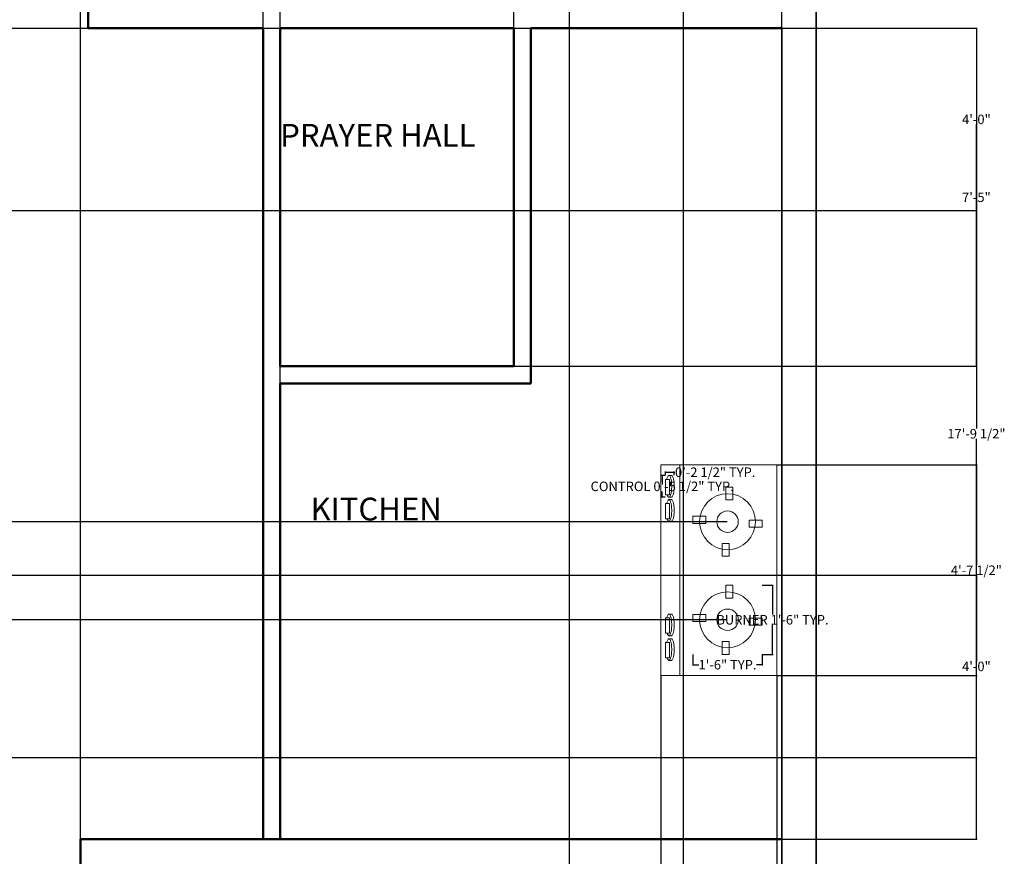
# Model space of a CAD drawing. Units: inches. Extents: x 594 to 1173, y 353 to 1285.
# Tile 5 of 6: x 914 to 1173, y 844 to 1065. Entities that reach past the tile are written whole.
import ezdxf

# ---------------------------------------------------------------- set-up
doc = ezdxf.new("R2010")
doc.units = ezdxf.units.IN
doc.header["$MEASUREMENT"] = 0
for name, color, linetype, lineweight in [('A-ANNO-DIMS', 2, 'Continuous', 18), ('A-AREA-IDEN', 7, 'Continuous', 25), ('A-EQPM', 8, 'Continuous', 18), ('A-WALL', 7, 'Continuous', 50), ('C-PROP', 7, 'Continuous', 35)]:
    doc.layers.add(name, color=color, linetype=linetype, lineweight=lineweight)
doc.styles.get("Standard").update_dxf_attribs({"font": 'arial.ttf'})
doc.dimstyles.get("Standard").update_dxf_attribs({"dimtxt": 2.5, "dimasz": 0.18, "dimexe": 0.18, "dimexo": 0.0625, "dimgap": 0.09, "dimtad": 0, "dimtih": 1, "dimtoh": 1, "dimzin": 0, "dimdsep": 46, "dimlunit": 3, "dimtxsty": 'Standard', "dimcen": 0.09, "dimadec": 0, "dimazin": 0, "dimtfac": 1, "dimtofl": 0, "dimtmove": 0, "dimatfit": 3, "dimfxl": 1, "dimtolj": 1, "dimtzin": 0, "dimarcsym": 0})

# ---------------------------------------------------------------- blocks, each defined once
blk = doc.blocks.new('COOKTOP-BURNER')
for p, q in [((-0.44, 9.1), (-0.44, 5.73)), ((1.43, 9.1), (-0.44, 9.1)), ((1.43, 5.73), (1.43, 9.1)), ((-0.44, 5.73), (1.43, 5.73)), ((-5.73, 1.43), (-9.1, 1.43)), ((-9.1, 1.43), (-9.1, -0.44)), ((-5.73, -0.44), (-5.73, 1.43)), ((5.73, 0.44), (5.73, -1.43)), ((9.1, 0.44), (5.73, 0.44)), ((9.1, -1.43), (9.1, 0.44)), ((-9.1, -0.44), (-5.73, -0.44)), ((5.73, -1.43), (9.1, -1.43)), ((-1.43, -5.73), (-1.43, -9.1)), ((0.44, -5.73), (-1.43, -5.73)), ((0.44, -9.1), (0.44, -5.73)), ((-1.43, -9.1), (0.44, -9.1))]:
    blk.add_line(p, q)
for radius in [7.35, 2.82]:
    blk.add_circle((0, 0), radius)
blk = doc.blocks.new('COOKTOP-CONTROL-KNOB')
for p, q in [((1.55, 5.72), (0.9, 5.72)), ((0, 0.65), (0, 4.69)), ((0, 4.69), (1.04, 4.69)), ((1.04, 4.69), (1.04, 0.65)), ((1.04, 0.65), (0, 0.65)), ((1.63, 0), (0.9, 0.01))]:
    blk.add_line(p, q)
for centre, radius, start, end in [((2.87, 4.24), 2.58, 148.0894, 165.5369), ((0.9, 5.47), 0.251, 90, 148.0894), ((0.9, 5.47), 0.251, 31.9106, 90), ((-1.08, 4.24), 2.58, 14.4631, 31.9106), ((1.55, 5.47), 0.251, 31.9106, 90), ((-0.42, 4.24), 2.58, 14.4631, 31.9106), ((6.08, 3.42), 5.89, 165.5369, 167.5389), ((-4.28, 3.42), 5.89, 6.0983, 14.4631), ((-9.43, 2.87), 11.07, 0, 6.0983), ((-9.43, 2.87), 11.07, 353.9017, 0), ((-3.62, 3.42), 5.89, 6.0983, 14.4631), ((-8.78, 2.87), 11.07, 0, 6.0983), ((-8.78, 2.87), 11.07, 353.9017, 0), ((2.87, 1.49), 2.58, 198.9155, 211.9106), ((0.9, 0.26), 0.251, 211.9106, 270), ((0.9, 0.26), 0.251, 270, 328.0894), ((-1.08, 1.49), 2.58, 328.0894, 345.5369), ((-4.28, 2.31), 5.89, 345.5369, 353.9017), ((1.55, 0.26), 0.251, 252.0546, 270), ((1.55, 0.26), 0.251, 270, 328.0894), ((-0.42, 1.49), 2.58, 328.0894, 345.5369), ((-3.62, 2.31), 5.89, 345.5369, 353.9017)]:
    blk.add_arc(centre, radius, start, end)
blk = doc.blocks.new('*D34')
at = {"layer": 'A-ANNO-DIMS', "color": 0, "lineweight": -2, "transparency": 16777216}
for p, q in [((1109.21, 915.65), (1112.06, 915.65)), ((1111.88, 915.47), (1111.88, 907.92)), ((1111.88, 897.63), (1111.88, 905.19)), ((1109.21, 897.45), (1112.06, 897.45))]:
    blk.add_line(p, q, dxfattribs=at)
at = {"layer": 'A-ANNO-DIMS', "color": 0, "transparency": 16777216}
for points in [[(1111.85, 915.47), (1111.91, 915.47), (1111.88, 915.65)], [(1111.85, 897.63), (1111.91, 897.63), (1111.88, 897.45)]]:
    blk.add_solid(points, dxfattribs=at)
at = {"layer": 'Defpoints', "color": 0, "transparency": 16777216}
for p in [(1109.15, 915.65), (1111.88, 915.65), (1109.15, 897.45)]:
    blk.add_point(p, dxfattribs=at)
at = {"layer": 'A-ANNO-DIMS', "color": 0, "transparency": 16777216, "insert": (1111.88, 906.55), "char_height": 2.5, "attachment_point": 5}
blk.add_mtext('\\A1;BURNER 1\'-6" TYP.', dxfattribs=at)
blk = doc.blocks.new('*D35')
at = {"layer": 'A-ANNO-DIMS', "color": 0, "lineweight": -2, "transparency": 16777216}
for p, q in [((1090.95, 897.39), (1090.95, 894.54)), ((1109.15, 897.39), (1109.15, 894.54)), ((1091.13, 894.72), (1092.46, 894.72)), ((1108.97, 894.72), (1107.64, 894.72))]:
    blk.add_line(p, q, dxfattribs=at)
at = {"layer": 'A-ANNO-DIMS', "color": 0, "transparency": 16777216}
for points in [[(1091.13, 894.75), (1091.13, 894.69), (1090.95, 894.72)], [(1108.97, 894.75), (1108.97, 894.69), (1109.15, 894.72)]]:
    blk.add_solid(points, dxfattribs=at)
at = {"layer": 'Defpoints', "color": 0, "transparency": 16777216}
for p in [(1090.95, 897.45), (1109.15, 897.45), (1109.15, 894.72)]:
    blk.add_point(p, dxfattribs=at)
at = {"layer": 'A-ANNO-DIMS', "color": 0, "transparency": 16777216, "insert": (1100.05, 894.72), "char_height": 2.5, "attachment_point": 5}
blk.add_mtext('\\A1;1\'-6" TYP.', dxfattribs=at)
blk = doc.blocks.new('*D36')
at = {"layer": 'A-ANNO-DIMS', "color": 0, "lineweight": -2, "transparency": 16777216}
for p, q in [((1083.66, 944.54), (1082.68, 944.54)), ((1082.86, 944.36), (1082.86, 943.07)), ((1083.66, 938.82), (1082.68, 938.82)), ((1082.86, 939), (1082.86, 940.3))]:
    blk.add_line(p, q, dxfattribs=at)
at = {"layer": 'A-ANNO-DIMS', "color": 0, "transparency": 16777216}
for points in [[(1082.83, 944.36), (1082.89, 944.36), (1082.86, 944.54)], [(1082.83, 939), (1082.89, 939), (1082.86, 938.82)]]:
    blk.add_solid(points, dxfattribs=at)
at = {"layer": 'Defpoints', "color": 0, "transparency": 16777216}
for p in [(1082.86, 944.54), (1083.72, 944.54), (1083.72, 938.82)]:
    blk.add_point(p, dxfattribs=at)
at = {"layer": 'A-ANNO-DIMS', "color": 0, "transparency": 16777216, "insert": (1082.86, 941.68), "char_height": 2.5, "attachment_point": 5}
blk.add_mtext('\\A1;CONTROL 0\'-5 1/2" TYP.', dxfattribs=at)
blk = doc.blocks.new('*D37')
at = {"layer": 'A-ANNO-DIMS', "color": 0, "lineweight": -2, "transparency": 16777216}
for p, q in [((1083.72, 944.61), (1083.72, 945.58)), ((1083.9, 945.4), (1085.83, 945.4)), ((1086.01, 944.61), (1086.01, 945.58)), ((1086.01, 945.4), (1086.19, 945.4))]:
    blk.add_line(p, q, dxfattribs=at)
at = {"layer": 'A-ANNO-DIMS', "color": 0, "transparency": 16777216}
for points in [[(1083.9, 945.43), (1083.9, 945.37), (1083.72, 945.4)], [(1085.83, 945.43), (1085.83, 945.37), (1086.01, 945.4)]]:
    blk.add_solid(points, dxfattribs=at)
at = {"layer": 'Defpoints', "color": 0, "transparency": 16777216}
for p in [(1083.72, 944.54), (1086.01, 945.4), (1086.01, 944.54)]:
    blk.add_point(p, dxfattribs=at)
at = {"layer": 'A-ANNO-DIMS', "color": 0, "transparency": 16777216, "insert": (1096.81, 945.4), "char_height": 2.5, "attachment_point": 5}
blk.add_mtext('\\A1;0\'-2 1/2" TYP.', dxfattribs=at)
blk = doc.blocks.new('*D52')
at = {"layer": 'A-ANNO-DIMS', "color": 0, "lineweight": -2, "transparency": 16777216}
for p, q in [((982.34, 968.85), (982.34, 1281.16)), ((982.52, 1280.98), (1044.07, 1280.98)), ((1114.16, 1280.98), (1052.6, 1280.98)), ((1114.34, 848.85), (1114.34, 1281.16))]:
    blk.add_line(p, q, dxfattribs=at)
at = {"layer": 'A-ANNO-DIMS', "color": 0, "transparency": 16777216}
for points in [[(982.52, 1281.01), (982.52, 1280.95), (982.34, 1280.98)], [(1114.16, 1281.01), (1114.16, 1280.95), (1114.34, 1280.98)]]:
    blk.add_solid(points, dxfattribs=at)
at = {"layer": 'Defpoints', "color": 0, "transparency": 16777216}
for p in [(1114.34, 1280.98), (982.34, 968.78), (1114.34, 848.78)]:
    blk.add_point(p, dxfattribs=at)
at = {"layer": 'A-ANNO-DIMS', "color": 0, "transparency": 16777216, "insert": (1048.34, 1280.98), "char_height": 2.5, "attachment_point": 5}
blk.add_mtext('\\A1;11\'-0"', dxfattribs=at)
blk = doc.blocks.new('*D53')
at = {"layer": 'A-ANNO-DIMS', "color": 0, "lineweight": -2, "transparency": 16777216}
for p, q in [((1114.4, 1062.28), (1165.72, 1062.28)), ((1165.54, 1062.1), (1165.54, 956.92)), ((1165.54, 848.96), (1165.54, 954.15)), ((1114.4, 848.78), (1165.72, 848.78))]:
    blk.add_line(p, q, dxfattribs=at)
at = {"layer": 'A-ANNO-DIMS', "color": 0, "transparency": 16777216}
for points in [[(1165.51, 1062.1), (1165.57, 1062.1), (1165.54, 1062.28)], [(1165.51, 848.96), (1165.57, 848.96), (1165.54, 848.78)]]:
    blk.add_solid(points, dxfattribs=at)
at = {"layer": 'Defpoints', "color": 0, "transparency": 16777216}
for p in [(1114.34, 1062.28), (1165.54, 1062.28), (1114.34, 848.78)]:
    blk.add_point(p, dxfattribs=at)
at = {"layer": 'A-ANNO-DIMS', "color": 0, "transparency": 16777216, "insert": (1165.54, 955.53), "char_height": 2.5, "attachment_point": 5}
blk.add_mtext('\\A1;17\'-9 1/2"', dxfattribs=at)
blk = doc.blocks.new('*D54')
at = {"layer": 'A-ANNO-DIMS', "color": 0, "lineweight": -2, "transparency": 16777216}
for p, q in [((982.34, 1062.35), (982.34, 1281.16)), ((982.52, 1280.98), (1006.76, 1280.98)), ((1043.66, 1280.98), (1019.41, 1280.98)), ((1043.84, 1062.35), (1043.84, 1281.16))]:
    blk.add_line(p, q, dxfattribs=at)
at = {"layer": 'A-ANNO-DIMS', "color": 0, "transparency": 16777216}
for points in [[(982.52, 1281.01), (982.52, 1280.95), (982.34, 1280.98)], [(1043.66, 1281.01), (1043.66, 1280.95), (1043.84, 1280.98)]]:
    blk.add_solid(points, dxfattribs=at)
at = {"layer": 'Defpoints', "color": 0, "transparency": 16777216}
for p in [(1043.84, 1280.98), (982.34, 1062.28), (1043.84, 1062.28)]:
    blk.add_point(p, dxfattribs=at)
at = {"layer": 'A-ANNO-DIMS', "color": 0, "transparency": 16777216, "insert": (1013.09, 1280.98), "char_height": 2.5, "attachment_point": 5}
blk.add_mtext('\\A1;5\'-1 1/2"', dxfattribs=at)
blk = doc.blocks.new('*D55')
at = {"layer": 'A-ANNO-DIMS', "color": 0, "lineweight": -2, "transparency": 16777216}
for p, q in [((1043.9, 1062.28), (1165.72, 1062.28)), ((1165.54, 1062.1), (1165.54, 1019.14)), ((1165.54, 973.46), (1165.54, 1016.42)), ((1043.9, 973.28), (1165.72, 973.28))]:
    blk.add_line(p, q, dxfattribs=at)
at = {"layer": 'A-ANNO-DIMS', "color": 0, "transparency": 16777216}
for points in [[(1165.51, 1062.1), (1165.57, 1062.1), (1165.54, 1062.28)], [(1165.51, 973.46), (1165.57, 973.46), (1165.54, 973.28)]]:
    blk.add_solid(points, dxfattribs=at)
at = {"layer": 'Defpoints', "color": 0, "transparency": 16777216}
for p in [(1043.84, 1062.28), (1165.54, 1062.28), (1043.84, 973.28)]:
    blk.add_point(p, dxfattribs=at)
at = {"layer": 'A-ANNO-DIMS', "color": 0, "transparency": 16777216, "insert": (1165.54, 1017.78), "char_height": 2.5, "attachment_point": 5}
blk.add_mtext('\\A1;7\'-5"', dxfattribs=at)
blk = doc.blocks.new('*D58')
at = {"layer": 'A-ANNO-DIMS', "color": 0, "lineweight": -2, "transparency": 16777216}
for p, q in [((829.34, 647.85), (829.34, 1281.16)), ((829.52, 1280.98), (873.26, 1280.98)), ((929.66, 1280.98), (885.91, 1280.98)), ((929.84, 647.85), (929.84, 1281.16))]:
    blk.add_line(p, q, dxfattribs=at)
at = {"layer": 'A-ANNO-DIMS', "color": 0, "transparency": 16777216}
for points in [[(829.52, 1281.01), (829.52, 1280.95), (829.34, 1280.98)], [(929.66, 1281.01), (929.66, 1280.95), (929.84, 1280.98)]]:
    blk.add_solid(points, dxfattribs=at)
at = {"layer": 'Defpoints', "color": 0, "transparency": 16777216}
for p in [(929.84, 1280.98), (829.34, 647.78), (929.84, 647.78)]:
    blk.add_point(p, dxfattribs=at)
at = {"layer": 'A-ANNO-DIMS', "color": 0, "transparency": 16777216, "insert": (879.59, 1280.98), "char_height": 2.5, "attachment_point": 5}
blk.add_mtext('\\A1;8\'-4 1/2"', dxfattribs=at)
blk = doc.blocks.new('*D61')
at = {"layer": 'A-ANNO-DIMS', "color": 0, "lineweight": -2, "transparency": 16777216}
for p, q in [((728.84, 1062.35), (728.84, 1281.16)), ((729.02, 1280.98), (848.93, 1280.98)), ((977.66, 1280.98), (857.74, 1280.98)), ((977.84, 1062.35), (977.84, 1281.16))]:
    blk.add_line(p, q, dxfattribs=at)
at = {"layer": 'A-ANNO-DIMS', "color": 0, "transparency": 16777216}
for points in [[(729.02, 1281.01), (729.02, 1280.95), (728.84, 1280.98)], [(977.66, 1281.01), (977.66, 1280.95), (977.84, 1280.98)]]:
    blk.add_solid(points, dxfattribs=at)
at = {"layer": 'Defpoints', "color": 0, "transparency": 16777216}
for p in [(977.84, 1280.98), (728.84, 1062.28), (977.84, 1062.28)]:
    blk.add_point(p, dxfattribs=at)
at = {"layer": 'A-ANNO-DIMS', "color": 0, "transparency": 16777216, "insert": (853.34, 1280.98), "char_height": 2.5, "attachment_point": 5}
blk.add_mtext('\\A1;20\'-9"', dxfattribs=at)
blk = doc.blocks.new('*D62')
at = {"layer": 'A-ANNO-DIMS', "color": 0, "lineweight": -2, "transparency": 16777216}
for p, q in [((1082.5, 891.79), (1082.5, 356.4)), ((1113.01, 891.79), (1113.01, 356.4)), ((1082.68, 356.58), (1091.41, 356.58)), ((1112.83, 356.58), (1104.1, 356.58))]:
    blk.add_line(p, q, dxfattribs=at)
at = {"layer": 'A-ANNO-DIMS', "color": 0, "transparency": 16777216}
for points in [[(1082.68, 356.61), (1082.68, 356.55), (1082.5, 356.58)], [(1112.83, 356.61), (1112.83, 356.55), (1113.01, 356.58)]]:
    blk.add_solid(points, dxfattribs=at)
at = {"layer": 'Defpoints', "color": 0, "transparency": 16777216}
for p in [(1082.5, 891.85), (1113.01, 891.85), (1113.01, 356.58)]:
    blk.add_point(p, dxfattribs=at)
at = {"layer": 'A-ANNO-DIMS', "color": 0, "transparency": 16777216, "insert": (1097.75, 356.58), "char_height": 2.5, "attachment_point": 5}
blk.add_mtext('\\A1;2\'-6 1/2"', dxfattribs=at)
blk = doc.blocks.new('*D63')
at = {"layer": 'A-ANNO-DIMS', "color": 0, "lineweight": -2, "transparency": 16777216}
for p, q in [((1113.07, 947.33), (1165.72, 947.33)), ((1165.54, 947.15), (1165.54, 920.97)), ((1165.54, 892.03), (1165.54, 918.21)), ((1113.07, 891.85), (1165.72, 891.85))]:
    blk.add_line(p, q, dxfattribs=at)
at = {"layer": 'A-ANNO-DIMS', "color": 0, "transparency": 16777216}
for points in [[(1165.51, 947.15), (1165.57, 947.15), (1165.54, 947.33)], [(1165.51, 892.03), (1165.57, 892.03), (1165.54, 891.85)]]:
    blk.add_solid(points, dxfattribs=at)
at = {"layer": 'Defpoints', "color": 0, "transparency": 16777216}
for p in [(1113.01, 947.33), (1165.54, 947.33), (1113.01, 891.85)]:
    blk.add_point(p, dxfattribs=at)
at = {"layer": 'A-ANNO-DIMS', "color": 0, "transparency": 16777216, "insert": (1165.54, 919.59), "char_height": 2.5, "attachment_point": 5}
blk.add_mtext('\\A1;4\'-7 1/2"', dxfattribs=at)
blk = doc.blocks.new('*D67')
at = {"layer": 'A-ANNO-DIMS', "color": 0, "lineweight": -2, "transparency": 16777216}
for p, q in [((1058.34, 1093.22), (1058.34, 356.4)), ((1088.34, 1093.22), (1088.34, 356.4)), ((1058.52, 356.58), (1069.9, 356.58)), ((1088.16, 356.58), (1076.77, 356.58))]:
    blk.add_line(p, q, dxfattribs=at)
at = {"layer": 'A-ANNO-DIMS', "color": 0, "transparency": 16777216}
for points in [[(1058.52, 356.61), (1058.52, 356.55), (1058.34, 356.58)], [(1088.16, 356.61), (1088.16, 356.55), (1088.34, 356.58)]]:
    blk.add_solid(points, dxfattribs=at)
at = {"layer": 'Defpoints', "color": 0, "transparency": 16777216}
for p in [(1058.34, 1093.28), (1088.34, 1093.28), (1058.34, 356.58)]:
    blk.add_point(p, dxfattribs=at)
at = {"layer": 'A-ANNO-DIMS', "color": 0, "transparency": 16777216, "insert": (1073.34, 356.58), "char_height": 2.5, "attachment_point": 5}
blk.add_mtext('\\A1;2\'-6"', dxfattribs=at)
blk = doc.blocks.new('*D71')
at = {"layer": 'A-ANNO-DIMS', "color": 0, "lineweight": -2, "transparency": 16777216}
for p, q in [((812.9, 918.28), (1165.72, 918.28)), ((1165.54, 918.1), (1165.54, 895.65)), ((1165.54, 870.46), (1165.54, 892.92)), ((812.9, 870.28), (1165.72, 870.28))]:
    blk.add_line(p, q, dxfattribs=at)
at = {"layer": 'A-ANNO-DIMS', "color": 0, "transparency": 16777216}
for points in [[(1165.51, 918.1), (1165.57, 918.1), (1165.54, 918.28)], [(1165.51, 870.46), (1165.57, 870.46), (1165.54, 870.28)]]:
    blk.add_solid(points, dxfattribs=at)
at = {"layer": 'Defpoints', "color": 0, "transparency": 16777216}
for p in [(812.84, 918.28), (1165.54, 918.28), (812.84, 870.28)]:
    blk.add_point(p, dxfattribs=at)
at = {"layer": 'A-ANNO-DIMS', "color": 0, "transparency": 16777216, "insert": (1165.54, 894.28), "char_height": 2.5, "attachment_point": 5}
blk.add_mtext('\\A1;4\'-0"', dxfattribs=at)
blk = doc.blocks.new('*D74')
at = {"layer": 'A-ANNO-DIMS', "color": 0, "lineweight": -2, "transparency": 16777216}
for p, q in [((812.9, 1062.28), (1165.72, 1062.28)), ((1165.54, 1062.1), (1165.54, 1039.65)), ((1165.54, 1014.46), (1165.54, 1036.92)), ((812.9, 1014.28), (1165.72, 1014.28))]:
    blk.add_line(p, q, dxfattribs=at)
at = {"layer": 'A-ANNO-DIMS', "color": 0, "transparency": 16777216}
for points in [[(1165.51, 1062.1), (1165.57, 1062.1), (1165.54, 1062.28)], [(1165.51, 1014.46), (1165.57, 1014.46), (1165.54, 1014.28)]]:
    blk.add_solid(points, dxfattribs=at)
at = {"layer": 'Defpoints', "color": 0, "transparency": 16777216}
for p in [(812.84, 1062.28), (1165.54, 1062.28), (812.84, 1014.28)]:
    blk.add_point(p, dxfattribs=at)
at = {"layer": 'A-ANNO-DIMS', "color": 0, "transparency": 16777216, "insert": (1165.54, 1038.28), "char_height": 2.5, "attachment_point": 5}
blk.add_mtext('\\A1;4\'-0"', dxfattribs=at)
blk = doc.blocks.new('*D79')
at = {"layer": 'A-ANNO-DIMS', "color": 0, "lineweight": -2, "transparency": 16777216}
for p, q in [((1099.99, 932.38), (600.96, 932.38)), ((601.14, 932.2), (601.14, 920.81)), ((601.14, 906.73), (601.14, 918.12)), ((1099.99, 906.55), (600.96, 906.55))]:
    blk.add_line(p, q, dxfattribs=at)
at = {"layer": 'A-ANNO-DIMS', "color": 0, "transparency": 16777216}
for points in [[(601.11, 932.2), (601.17, 932.2), (601.14, 932.38)], [(601.11, 906.73), (601.17, 906.73), (601.14, 906.55)]]:
    blk.add_solid(points, dxfattribs=at)
at = {"layer": 'Defpoints', "color": 0, "transparency": 16777216}
for p in [(601.14, 932.38), (1100.05, 932.38), (1100.05, 906.55)]:
    blk.add_point(p, dxfattribs=at)
at = {"layer": 'A-ANNO-DIMS', "color": 0, "transparency": 16777216, "insert": (601.14, 919.47), "char_height": 2.5, "attachment_point": 5}
blk.add_mtext('\\A1;2\'-2"', dxfattribs=at)

msp = doc.modelspace()

# ---------------------------------------------------------------- linework, layer by layer
at = {"layer": 'A-EQPM'}
for p, q in [((1082.501, 947.329), (1113.008, 947.329)), ((1082.501, 891.849), (1082.501, 947.329)), ((1087.463, 891.849), (1087.463, 947.329)), ((1113.008, 947.329), (1113.008, 891.849)), ((1113.008, 891.849), (1082.501, 891.849))]:
    msp.add_line(p, q, dxfattribs=at)
at = {"layer": 'A-WALL'}
for p, q in [((931.837, 1062.283), (931.837, 1066.783)), ((931.837, 1062.283), (977.837, 1062.283)), ((977.837, 848.783), (977.837, 1062.283)), ((982.337, 973.283), (982.337, 1062.283)), ((982.337, 1062.283), (1043.837, 1062.283)), ((1043.837, 973.283), (1043.837, 1062.283)), ((1048.337, 968.783), (1048.337, 1062.283)), ((1048.337, 1062.283), (1114.337, 1062.283)), ((982.337, 973.283), (1043.837, 973.283)), ((982.337, 848.783), (982.337, 968.783)), ((982.337, 968.783), (1048.337, 968.783)), ((929.837, 848.783), (1114.337, 848.783)), ((929.837, 835.783), (929.837, 848.783))]:
    msp.add_line(p, q, dxfattribs=at)
at = {"layer": 'C-PROP'}
for p, q in [((1123.337, 398.783), (1123.337, 1238.783)), ((1114.337, 407.783), (1114.337, 1062.283))]:
    msp.add_line(p, q, dxfattribs=at)

# ---------------------------------------------------------------- block references
at = {"layer": 'A-EQPM'}
for name, p in [('COOKTOP-CONTROL-KNOB', (1083.721, 938.821)), ('COOKTOP-BURNER', (1100.051, 932.38)), ('COOKTOP-CONTROL-KNOB', (1083.721, 932.458)), ('COOKTOP-BURNER', (1100.051, 906.552)), ('COOKTOP-CONTROL-KNOB', (1083.721, 902.338)), ('COOKTOP-CONTROL-KNOB', (1083.721, 895.85))]:
    msp.add_blockref(name, p, dxfattribs=at)

# ---------------------------------------------------------------- texts
at = {"layer": 'A-AREA-IDEN'}
for s, p in [('PRAYER HALL', (982.337, 1031.093)), ('KITCHEN', (990.339, 932.695))]:
    msp.add_text(s, height=6, dxfattribs=at).set_placement(p)

# ---------------------------------------------------------------- dimensions: what is measured, and where the dimension line sits
at = {"layer": 'A-ANNO-DIMS'}
for base, p1, p2, picture, middle in [((977.837, 1280.983), (728.837, 1062.283), (977.837, 1062.283), '*D61', (853.337, 1280.983)), ((929.837, 1280.983), (829.337, 647.783), (929.837, 647.783), '*D58', (879.587, 1280.983)), ((1043.837, 1280.983), (982.337, 1062.283), (1043.837, 1062.283), '*D54', (1013.087, 1280.983)), ((1114.337, 1280.983), (982.337, 968.783), (1114.337, 848.783), '*D52', (1048.337, 1280.983)), ((1058.337, 356.583), (1088.337, 1093.283), (1058.337, 1093.283), '*D67', (1073.337, 356.583)), ((1113.008, 356.583), (1082.501, 891.849), (1113.008, 891.849), '*D62', (1097.755, 356.583))]:
    dim = msp.add_linear_dim(base=base, p1=p1, p2=p2, dimstyle='Standard', override={"dimdec": 1, "dimlfac": 1, "dimrnd": 0, "dimzin": 1, "dimdsep": 46, "dimlunit": 4, "dimfrac": 2}, dxfattribs=at)
    dim.commit()
    dim.dimension.update_dxf_attribs({"geometry": picture, "text_midpoint": middle})
for base, p1, p2, picture, middle in [((1165.537, 1062.283), (812.837, 1014.283), (812.837, 1062.283), '*D74', (1165.537, 1038.283)), ((1165.537, 1062.283), (1043.837, 973.283), (1043.837, 1062.283), '*D55', (1165.537, 1017.783)), ((1165.537, 1062.283), (1114.337, 848.783), (1114.337, 1062.283), '*D53', (1165.537, 955.533)), ((1165.537, 947.329), (1113.008, 891.849), (1113.008, 947.329), '*D63', (1165.537, 919.589)), ((601.137, 932.38), (1100.051, 906.552), (1100.051, 932.38), '*D79', (601.137, 919.466)), ((1165.537, 918.283), (812.837, 870.283), (812.837, 918.283), '*D71', (1165.537, 894.283))]:
    dim = msp.add_linear_dim(base=base, p1=p1, p2=p2, angle=90, dimstyle='Standard', override={"dimdec": 1, "dimlfac": 1, "dimrnd": 0, "dimzin": 1, "dimdsep": 46, "dimlunit": 4, "dimfrac": 2}, dxfattribs=at)
    dim.commit()
    dim.dimension.update_dxf_attribs({"geometry": picture, "text_midpoint": middle})
for base, p1, p2, picture, middle in [((1086.012, 945.402), (1083.721, 944.544), (1086.012, 944.544), '*D37', (1096.814, 945.402)), ((1109.149, 894.724), (1090.952, 897.453), (1109.149, 897.453), '*D35', (1100.051, 894.724))]:
    dim = msp.add_linear_dim(base=base, p1=p1, p2=p2, text='<> TYP.', dimstyle='Standard', override={"dimdec": 1, "dimlfac": 1, "dimrnd": 0, "dimzin": 1, "dimdsep": 46, "dimlunit": 4, "dimfrac": 2}, dxfattribs=at)
    dim.commit()
    dim.dimension.update_dxf_attribs({"geometry": picture, "text_midpoint": middle})
for base, p1, p2, text, picture, middle in [((1082.863, 944.544), (1083.721, 938.822), (1083.721, 944.544), 'CONTROL <> TYP.', '*D36', (1082.863, 941.683)), ((1111.879, 915.651), (1109.149, 897.453), (1109.149, 915.651), 'BURNER <> TYP.', '*D34', (1111.879, 906.552))]:
    dim = msp.add_linear_dim(base=base, p1=p1, p2=p2, angle=90, text=text, dimstyle='Standard', override={"dimdec": 1, "dimlfac": 1, "dimrnd": 0, "dimzin": 1, "dimdsep": 46, "dimlunit": 4, "dimfrac": 2}, dxfattribs=at)
    dim.commit()
    dim.dimension.update_dxf_attribs({"geometry": picture, "text_midpoint": middle})

doc.saveas('drawing.dxf')
